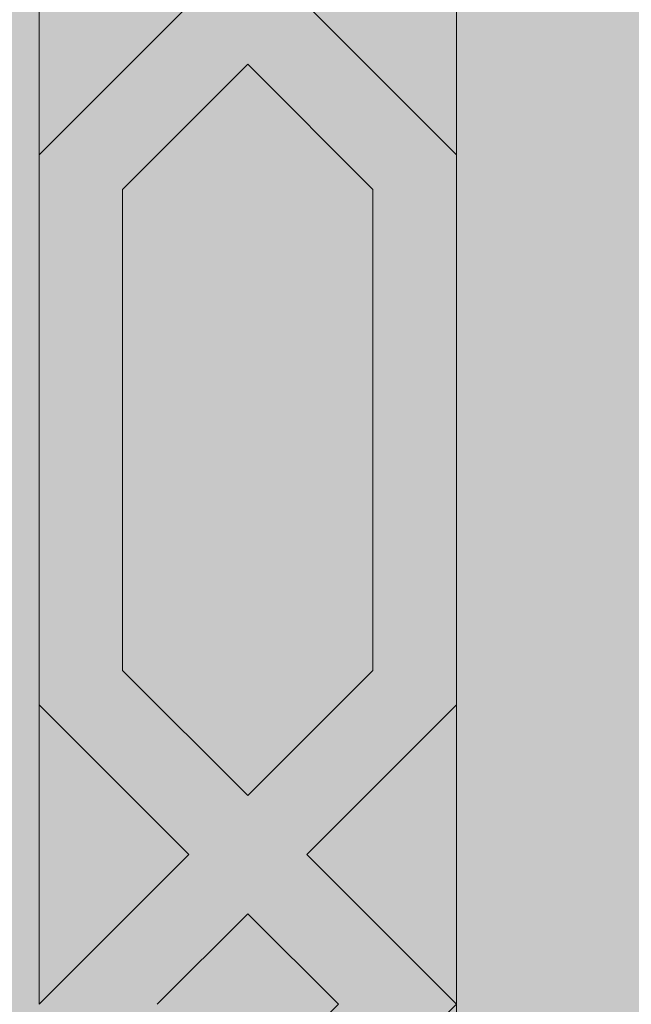
# Model space of a CAD drawing. Units: inches. Extents: x 844 to 2234, y 346 to 1084.
# Tile 14 of 93: x 1116.421 to 1118.29, y 696.22 to 699.229. Entities that reach past the tile are written whole.
import ezdxf

# ---------------------------------------------------------------- set-up
doc = ezdxf.new("R2010")
doc.units = ezdxf.units.IN
doc.header["$MEASUREMENT"] = 0
for name, color, linetype, lineweight in [('A-ANNO-DIMS', 2, 'Continuous', 18), ('furniture', 8, 'Continuous', 18), ('RA-AP-01$0$INT', 35, 'Continuous', 5)]:
    doc.layers.add(name, color=color, linetype=linetype, lineweight=lineweight)
doc.layers.add('RA-AP-01$0$FURN', color=3, linetype='Continuous')
doc.styles.get("Standard").update_dxf_attribs({"font": 'arial.ttf'})
doc.dimstyles.get("Standard").update_dxf_attribs({"dimtxt": 6, "dimasz": 3, "dimexe": 0.18, "dimexo": 0.0625, "dimgap": 0.09, "dimtad": 0, "dimtih": 1, "dimtoh": 1, "dimdec": 1, "dimzin": 0, "dimdsep": 46, "dimlunit": 3, "dimtxsty": 'Standard', "dimblk": 'ARCHTICK', "dimcen": 0.09, "dimadec": 0, "dimazin": 0, "dimtfac": 1, "dimtdec": 1, "dimtofl": 0, "dimtmove": 0, "dimatfit": 3, "dimfxl": 1, "dimtolj": 1, "dimtzin": 0, "dimarcsym": 0})

# ---------------------------------------------------------------- blocks, each defined once
blk = doc.blocks.new('A$C18D01794')
at = {"layer": 'RA-AP-01$0$INT'}
h = blk.add_hatch(color=256, dxfattribs=at)
h.paths.add_polyline_path([(4.35521, -6.15671), (4.35521, -8.05671), (5.45521, -8.05671), (5.45521, -6.15671)])
h.paths.add_polyline_path([(4.40521, -8.00671), (4.40521, -6.20671), (5.40521, -6.20671), (5.40521, -8.00671)], flags=16)
h = blk.add_hatch(color=256, dxfattribs=at)
h.paths.add_polyline_path([(4.46935, -7.07085), (4.50521, -7.035), (4.50521, -7.10671)])
h.paths.add_polyline_path([(4.45521, -7.085), (4.47692, -7.10671), (4.43349, -7.10671)])
h.paths.add_polyline_path([(4.40521, -7.035), (4.44106, -7.07085), (4.40521, -7.10671)])
h.paths.add_polyline_path([(4.42521, -6.91146), (4.45521, -6.88146), (4.48521, -6.91146), (4.48521, -7.02671), (4.45521, -7.05671), (4.42521, -7.02671)])
h.paths.add_polyline_path([(4.50521, -6.83146), (4.50521, -6.90318), (4.46935, -6.86732)])
h.paths.add_polyline_path([(4.42521, -6.70793), (4.45521, -6.67793), (4.48521, -6.70793), (4.48521, -6.82318), (4.45521, -6.85318), (4.42521, -6.82318)])
h.paths.add_polyline_path([(4.42521, -6.50439), (4.45521, -6.47439), (4.48521, -6.50439), (4.48521, -6.61964), (4.45521, -6.64964), (4.42521, -6.61964)])
h.paths.add_polyline_path([(4.46935, -6.66378), (4.50521, -6.62793), (4.50521, -6.69964)])
h.paths.add_polyline_path([(4.40521, -6.62793), (4.44106, -6.66378), (4.40521, -6.69964)])
h.paths.add_polyline_path([(4.40521, -6.42439), (4.44106, -6.46025), (4.40521, -6.49611)])
h.paths.add_polyline_path([(4.46935, -6.46025), (4.50521, -6.42439), (4.50521, -6.49611)])
h.paths.add_polyline_path([(4.42521, -6.30085), (4.45521, -6.27085), (4.48521, -6.30085), (4.48521, -6.41611), (4.45521, -6.44611), (4.42521, -6.41611)])
h.paths.add_polyline_path([(4.42521, -6.22671), (4.47106, -6.22671), (4.42521, -6.27257)])
h.paths.add_polyline_path([(4.49935, -6.22671), (4.63606, -6.22671), (4.66606, -6.25671), (4.63606, -6.28671), (4.49935, -6.28671), (4.46935, -6.25671)])
h.paths.add_polyline_path([(4.68021, -6.27085), (4.71606, -6.30671), (4.64435, -6.30671)])
h.paths.add_polyline_path([(4.64435, -6.20671), (4.71606, -6.20671), (4.68021, -6.24257)])
h.paths.add_polyline_path([(4.72435, -6.22671), (4.86106, -6.22671), (4.89106, -6.25671), (4.86106, -6.28671), (4.72435, -6.28671), (4.69435, -6.25671)])
h.paths.add_polyline_path([(4.90521, -6.27085), (4.94106, -6.30671), (4.86935, -6.30671)])
h.paths.add_polyline_path([(4.86935, -6.20671), (4.94106, -6.20671), (4.90521, -6.24257)])
h.paths.add_polyline_path([(4.94935, -6.22671), (5.08606, -6.22671), (5.11606, -6.25671), (5.08606, -6.28671), (4.94935, -6.28671), (4.91935, -6.25671)])
h.paths.add_polyline_path([(5.13021, -6.27085), (5.16606, -6.30671), (5.09435, -6.30671)])
h.paths.add_polyline_path([(5.09435, -6.20671), (5.16606, -6.20671), (5.13021, -6.24257)])
h.paths.add_polyline_path([(5.17435, -6.22671), (5.31106, -6.22671), (5.34106, -6.25671), (5.31106, -6.28671), (5.17435, -6.28671), (5.14435, -6.25671)])
h.paths.add_polyline_path([(5.32521, -6.30085), (5.35521, -6.27085), (5.38521, -6.30085), (5.38521, -6.41611), (5.35521, -6.44611), (5.32521, -6.41611)])
h.paths.add_polyline_path([(5.33935, -6.22671), (5.38521, -6.22671), (5.38521, -6.27257)])
h.paths.add_polyline_path([(5.32521, -6.50439), (5.35521, -6.47439), (5.38521, -6.50439), (5.38521, -6.61964), (5.35521, -6.64964), (5.32521, -6.61964)])
h.paths.add_polyline_path([(5.30521, -6.42439), (5.34106, -6.46025), (5.30521, -6.49611)])
h.paths.add_polyline_path([(5.36935, -6.46025), (5.40521, -6.42439), (5.40521, -6.49611)])
h.paths.add_polyline_path([(5.40521, -6.62793), (5.40521, -6.69964), (5.36935, -6.66378)])
h.paths.add_polyline_path([(5.30521, -6.62793), (5.34106, -6.66378), (5.30521, -6.69964)])
h.paths.add_polyline_path([(5.32521, -6.70793), (5.35521, -6.67793), (5.38521, -6.70793), (5.38521, -6.82318), (5.35521, -6.85318), (5.32521, -6.82318)])
h.paths.add_polyline_path([(5.30521, -6.83146), (5.34106, -6.86732), (5.30521, -6.90318)])
h.paths.add_polyline_path([(5.32521, -6.91146), (5.35521, -6.88146), (5.38521, -6.91146), (5.38521, -7.02671), (5.35521, -7.05671), (5.32521, -7.02671)])
h.paths.add_polyline_path([(5.40458, -6.83209, 0.001218), (5.40521, -6.83231), (5.40521, -6.90318), (5.36935, -6.86732)])
h.paths.add_polyline_path([(5.36935, -7.07085), (5.40521, -7.035), (5.40521, -7.10671)])
h.paths.add_polyline_path([(5.35521, -7.085), (5.37692, -7.10671), (5.33349, -7.10671)])
h.paths.add_polyline_path([(5.30521, -7.035), (5.34106, -7.07085), (5.30521, -7.10671)])
h = blk.add_hatch(color=256, dxfattribs=at)
h.paths.add_polyline_path([(4.50521, -6.62793), (4.46935, -6.66378), (4.50521, -6.69964), (4.50521, -6.83146), (4.46935, -6.86732), (4.50521, -6.90318), (4.50521, -7.035), (4.46935, -7.07085), (4.50521, -7.10671), (4.47692, -7.10671), (4.45521, -7.085), (4.43349, -7.10671), (4.40521, -7.10671), (4.44106, -7.07085), (4.40521, -7.035), (4.40521, -6.90318), (4.44106, -6.86732), (4.40521, -6.83146), (4.40521, -6.69964), (4.44106, -6.66378), (4.40521, -6.62793), (4.40521, -6.49611), (4.44106, -6.46025), (4.40521, -6.42439), (4.40521, -6.20671), (4.64435, -6.20671), (4.68021, -6.24257), (4.71606, -6.20671), (4.86935, -6.20671), (4.90521, -6.24257), (4.94106, -6.20671), (5.09435, -6.20671), (5.13021, -6.24257), (5.16606, -6.20671), (5.40521, -6.20671), (5.40521, -6.42439), (5.36935, -6.46025), (5.40521, -6.49611), (5.40521, -6.62793), (5.36935, -6.66378), (5.40521, -6.69964), (5.40521, -6.83146), (5.36935, -6.86732), (5.40521, -6.90318), (5.40521, -7.035), (5.36935, -7.07085), (5.40521, -7.10671), (5.37692, -7.10671), (5.35521, -7.085), (5.33349, -7.10671), (5.30521, -7.10671), (5.34106, -7.07085), (5.30521, -7.035), (5.30521, -6.90318), (5.34106, -6.86732), (5.30521, -6.83146), (5.30521, -6.69964), (5.34106, -6.66378), (5.30521, -6.62793), (5.30521, -6.49611), (5.34106, -6.46025), (5.30521, -6.42439), (5.30521, -6.30671), (5.16606, -6.30671), (5.13021, -6.27085), (5.09435, -6.30671), (4.94106, -6.30671), (4.90521, -6.27085), (4.86935, -6.30671), (4.71606, -6.30671), (4.68021, -6.27085), (4.64435, -6.30671), (4.50521, -6.30671), (4.50521, -6.42439), (4.46935, -6.46025), (4.50521, -6.49611)])
h.paths.add_polyline_path([(4.48521, -6.50439), (4.45521, -6.47439), (4.42521, -6.50439), (4.42521, -6.61964), (4.45521, -6.64964), (4.48521, -6.61964)], flags=16)
h.paths.add_polyline_path([(4.45521, -6.44611), (4.48521, -6.41611), (4.48521, -6.30085), (4.45521, -6.27085), (4.42521, -6.30085), (4.42521, -6.41611)], flags=16)
h.paths.add_polyline_path([(4.45521, -6.67793), (4.42521, -6.70793), (4.42521, -6.82318), (4.45521, -6.85318), (4.48521, -6.82318), (4.48521, -6.70793)], flags=16)
h.paths.add_polyline_path([(4.49935, -6.28671), (4.63606, -6.28671), (4.66606, -6.25671), (4.63606, -6.22671), (4.49935, -6.22671), (4.46935, -6.25671)], flags=16)
h.paths.add_polyline_path([(4.42521, -6.27257), (4.47106, -6.22671), (4.42521, -6.22671)], flags=16)
h.paths.add_polyline_path([(4.45521, -6.88146), (4.42521, -6.91146), (4.42521, -7.02671), (4.45521, -7.05671), (4.48521, -7.02671), (4.48521, -6.91146)], flags=16)
h.paths.add_polyline_path([(4.72435, -6.28671), (4.86106, -6.28671), (4.89106, -6.25671), (4.86106, -6.22671), (4.72435, -6.22671), (4.69435, -6.25671)], flags=16)
h.paths.add_polyline_path([(4.91935, -6.25671), (4.94935, -6.28671), (5.08606, -6.28671), (5.11606, -6.25671), (5.08606, -6.22671), (4.94935, -6.22671)], flags=16)
h.paths.add_polyline_path([(5.14435, -6.25671), (5.17435, -6.28671), (5.31106, -6.28671), (5.34106, -6.25671), (5.31106, -6.22671), (5.17435, -6.22671)], flags=16)
h.paths.add_polyline_path([(5.32521, -6.61964), (5.35521, -6.64964), (5.38521, -6.61964), (5.38521, -6.50439), (5.35521, -6.47439), (5.32521, -6.50439)], flags=16)
h.paths.add_polyline_path([(5.32521, -6.41611), (5.35521, -6.44611), (5.38521, -6.41611), (5.38521, -6.30085), (5.35521, -6.27085), (5.32521, -6.30085)], flags=16)
h.paths.add_polyline_path([(5.32521, -6.70793), (5.32521, -6.82318), (5.35521, -6.85318), (5.38521, -6.82318), (5.38521, -6.70793), (5.35521, -6.67793)], flags=16)
h.paths.add_polyline_path([(5.32521, -6.91146), (5.32521, -7.02671), (5.35521, -7.05671), (5.38521, -7.02671), (5.38521, -6.91146), (5.35521, -6.88146)], flags=16)
h.paths.add_polyline_path([(5.33935, -6.22671), (5.38521, -6.27257), (5.38521, -6.22671)], flags=16)
for points in [[(4.50521, -6.30671), (5.30521, -6.30671), (5.30521, -7.10671), (5.25521, -7.10671), (5.25521, -6.35671), (4.55521, -6.35671), (4.55521, -7.10671), (4.50521, -7.10671)], [(4.50521, -7.90671), (5.30521, -7.90671), (5.30521, -7.10671), (5.25521, -7.10671), (5.25521, -7.85671), (4.55521, -7.85671), (4.55521, -7.10671), (4.50521, -7.10671)], [(4.40521, -7.38196), (4.44106, -7.34611), (4.40521, -7.31025)]]:
    blk.add_hatch(color=256, dxfattribs=at).paths.add_polyline_path(points)
h = blk.add_hatch(color=256, dxfattribs=at)
h.paths.add_polyline_path([(4.50521, -7.5855), (4.46935, -7.54964), (4.50521, -7.51378), (4.50521, -7.38196), (4.46935, -7.34611), (4.50521, -7.31025), (4.50521, -7.17843), (4.46935, -7.14257), (4.50521, -7.10671), (4.47692, -7.10671), (4.45521, -7.12843), (4.43349, -7.10671), (4.40521, -7.10671), (4.44106, -7.14257), (4.40521, -7.17843), (4.40521, -7.31025), (4.44106, -7.34611), (4.40521, -7.38196), (4.40521, -7.51378), (4.44106, -7.54964), (4.40521, -7.5855), (4.40521, -7.71732), (4.44106, -7.75318), (4.40521, -7.78903), (4.40521, -8.00671), (4.64435, -8.00671), (4.68021, -7.97085), (4.71606, -8.00671), (4.86935, -8.00671), (4.90521, -7.97085), (4.94106, -8.00671), (5.09435, -8.00671), (5.13021, -7.97085), (5.16606, -8.00671), (5.40521, -8.00671), (5.40521, -7.78903), (5.36935, -7.75318), (5.40521, -7.71732), (5.40521, -7.5855), (5.36935, -7.54964), (5.40521, -7.51378), (5.40521, -7.38196), (5.36935, -7.34611), (5.40521, -7.31025), (5.40521, -7.17843), (5.36935, -7.14257), (5.40521, -7.10671), (5.37692, -7.10671), (5.35521, -7.12843), (5.33349, -7.10671), (5.30521, -7.10671), (5.34106, -7.14257), (5.30521, -7.17843), (5.30521, -7.31025), (5.34106, -7.34611), (5.30521, -7.38196), (5.30521, -7.51378), (5.34106, -7.54964), (5.30521, -7.5855), (5.30521, -7.71732), (5.34106, -7.75318), (5.30521, -7.78903), (5.30521, -7.90671), (5.16606, -7.90671), (5.13021, -7.94257), (5.09435, -7.90671), (4.94106, -7.90671), (4.90521, -7.94257), (4.86935, -7.90671), (4.71606, -7.90671), (4.68021, -7.94257), (4.64435, -7.90671), (4.50521, -7.90671), (4.50521, -7.78903), (4.46935, -7.75318), (4.50521, -7.71732)])
h.paths.add_polyline_path([(4.48521, -7.70903), (4.45521, -7.73903), (4.42521, -7.70903), (4.42521, -7.59378), (4.45521, -7.56378), (4.48521, -7.59378)], flags=16)
h.paths.add_polyline_path([(4.45521, -7.76732), (4.48521, -7.79732), (4.48521, -7.91257), (4.45521, -7.94257), (4.42521, -7.91257), (4.42521, -7.79732)], flags=16)
h.paths.add_polyline_path([(4.45521, -7.5355), (4.42521, -7.5055), (4.42521, -7.39025), (4.45521, -7.36025), (4.48521, -7.39025), (4.48521, -7.5055)], flags=16)
h.paths.add_polyline_path([(4.49935, -7.92671), (4.63606, -7.92671), (4.66606, -7.95671), (4.63606, -7.98671), (4.49935, -7.98671), (4.46935, -7.95671)], flags=16)
h.paths.add_polyline_path([(4.42521, -7.94085), (4.47106, -7.98671), (4.42521, -7.98671)], flags=16)
h.paths.add_polyline_path([(4.45521, -7.33196), (4.42521, -7.30196), (4.42521, -7.18671), (4.45521, -7.15671), (4.48521, -7.18671), (4.48521, -7.30196)], flags=16)
h.paths.add_polyline_path([(4.72435, -7.92671), (4.86106, -7.92671), (4.89106, -7.95671), (4.86106, -7.98671), (4.72435, -7.98671), (4.69435, -7.95671)], flags=16)
h.paths.add_polyline_path([(4.91935, -7.95671), (4.94935, -7.92671), (5.08606, -7.92671), (5.11606, -7.95671), (5.08606, -7.98671), (4.94935, -7.98671)], flags=16)
h.paths.add_polyline_path([(5.14435, -7.95671), (5.17435, -7.92671), (5.31106, -7.92671), (5.34106, -7.95671), (5.31106, -7.98671), (5.17435, -7.98671)], flags=16)
h.paths.add_polyline_path([(5.32521, -7.59378), (5.35521, -7.56378), (5.38521, -7.59378), (5.38521, -7.70903), (5.35521, -7.73903), (5.32521, -7.70903)], flags=16)
h.paths.add_polyline_path([(5.32521, -7.79732), (5.35521, -7.76732), (5.38521, -7.79732), (5.38521, -7.91257), (5.35521, -7.94257), (5.32521, -7.91257)], flags=16)
h.paths.add_polyline_path([(5.32521, -7.5055), (5.32521, -7.39025), (5.35521, -7.36025), (5.38521, -7.39025), (5.38521, -7.5055), (5.35521, -7.5355)], flags=16)
h.paths.add_polyline_path([(5.32521, -7.30196), (5.32521, -7.18671), (5.35521, -7.15671), (5.38521, -7.18671), (5.38521, -7.30196), (5.35521, -7.33196)], flags=16)
h.paths.add_polyline_path([(5.33935, -7.98671), (5.38521, -7.94085), (5.38521, -7.98671)], flags=16)
h = blk.add_hatch(color=256, dxfattribs=at)
h.paths.add_polyline_path([(4.46935, -7.14257), (4.50521, -7.17843), (4.50521, -7.10671)])
h.paths.add_polyline_path([(4.45521, -7.12843), (4.47692, -7.10671), (4.43349, -7.10671)])
h.paths.add_polyline_path([(4.40521, -7.17843), (4.44106, -7.14257), (4.40521, -7.10671)])
h.paths.add_polyline_path([(4.42521, -7.30196), (4.45521, -7.33196), (4.48521, -7.30196), (4.48521, -7.18671), (4.45521, -7.15671), (4.42521, -7.18671)])
h.paths.add_polyline_path([(4.50521, -7.38196), (4.50521, -7.31025), (4.46935, -7.34611)])
h.paths.add_polyline_path([(4.42521, -7.5055), (4.45521, -7.5355), (4.48521, -7.5055), (4.48521, -7.39025), (4.45521, -7.36025), (4.42521, -7.39025)])
h.paths.add_polyline_path([(4.42521, -7.70903), (4.45521, -7.73903), (4.48521, -7.70903), (4.48521, -7.59378), (4.45521, -7.56378), (4.42521, -7.59378)])
h.paths.add_polyline_path([(4.46935, -7.54964), (4.50521, -7.5855), (4.50521, -7.51378)])
h.paths.add_polyline_path([(4.40521, -7.5855), (4.44106, -7.54964), (4.40521, -7.51378)])
h.paths.add_polyline_path([(4.40521, -7.78903), (4.44106, -7.75318), (4.40521, -7.71732)])
h.paths.add_polyline_path([(4.46935, -7.75318), (4.50521, -7.78903), (4.50521, -7.71732)])
h.paths.add_polyline_path([(4.42521, -7.91257), (4.45521, -7.94257), (4.48521, -7.91257), (4.48521, -7.79732), (4.45521, -7.76732), (4.42521, -7.79732)])
h.paths.add_polyline_path([(4.42521, -7.98671), (4.47106, -7.98671), (4.42521, -7.94085)])
h.paths.add_polyline_path([(4.49935, -7.98671), (4.63606, -7.98671), (4.66606, -7.95671), (4.63606, -7.92671), (4.49935, -7.92671), (4.46935, -7.95671)])
h.paths.add_polyline_path([(4.68021, -7.94257), (4.71606, -7.90671), (4.64435, -7.90671)])
h.paths.add_polyline_path([(4.64435, -8.00671), (4.71606, -8.00671), (4.68021, -7.97085)])
h.paths.add_polyline_path([(4.72435, -7.98671), (4.86106, -7.98671), (4.89106, -7.95671), (4.86106, -7.92671), (4.72435, -7.92671), (4.69435, -7.95671)])
h.paths.add_polyline_path([(4.90521, -7.94257), (4.94106, -7.90671), (4.86935, -7.90671)])
h.paths.add_polyline_path([(4.86935, -8.00671), (4.94106, -8.00671), (4.90521, -7.97085)])
h.paths.add_polyline_path([(4.94935, -7.98671), (5.08606, -7.98671), (5.11606, -7.95671), (5.08606, -7.92671), (4.94935, -7.92671), (4.91935, -7.95671)])
h.paths.add_polyline_path([(5.13021, -7.94257), (5.16606, -7.90671), (5.09435, -7.90671)])
h.paths.add_polyline_path([(5.09435, -8.00671), (5.16606, -8.00671), (5.13021, -7.97085)])
h.paths.add_polyline_path([(5.17435, -7.98671), (5.31106, -7.98671), (5.34106, -7.95671), (5.31106, -7.92671), (5.17435, -7.92671), (5.14435, -7.95671)])
h.paths.add_polyline_path([(5.32521, -7.91257), (5.35521, -7.94257), (5.38521, -7.91257), (5.38521, -7.79732), (5.35521, -7.76732), (5.32521, -7.79732)])
h.paths.add_polyline_path([(5.33935, -7.98671), (5.38521, -7.98671), (5.38521, -7.94085)])
h.paths.add_polyline_path([(5.32521, -7.70903), (5.35521, -7.73903), (5.38521, -7.70903), (5.38521, -7.59378), (5.35521, -7.56378), (5.32521, -7.59378)])
h.paths.add_polyline_path([(5.30521, -7.78903), (5.34106, -7.75318), (5.30521, -7.71732)])
h.paths.add_polyline_path([(5.36935, -7.75318), (5.40521, -7.78903), (5.40521, -7.71732)])
h.paths.add_polyline_path([(5.40521, -7.5855), (5.40521, -7.51378), (5.36935, -7.54964)])
h.paths.add_polyline_path([(5.30521, -7.5855), (5.34106, -7.54964), (5.30521, -7.51378)])
h.paths.add_polyline_path([(5.32521, -7.5055), (5.35521, -7.5355), (5.38521, -7.5055), (5.38521, -7.39025), (5.35521, -7.36025), (5.32521, -7.39025)])
h.paths.add_polyline_path([(5.30521, -7.38196), (5.34106, -7.34611), (5.30521, -7.31025)])
h.paths.add_polyline_path([(5.32521, -7.30196), (5.35521, -7.33196), (5.38521, -7.30196), (5.38521, -7.18671), (5.35521, -7.15671), (5.32521, -7.18671)])
h.paths.add_polyline_path([(5.40458, -7.38134, -0.001218), (5.40521, -7.38111), (5.40521, -7.31025), (5.36935, -7.34611)])
h.paths.add_polyline_path([(5.36935, -7.14257), (5.40521, -7.17843), (5.40521, -7.10671)])
h.paths.add_polyline_path([(5.35521, -7.12843), (5.37692, -7.10671), (5.33349, -7.10671)])
h.paths.add_polyline_path([(5.30521, -7.17843), (5.34106, -7.14257), (5.30521, -7.10671)])
for p, q in [((4.46935, -7.07085), (4.50521, -7.10671)), ((4.45521, -7.085), (4.47692, -7.10671)), ((4.44106, -7.14257), (4.40521, -7.10671)), ((4.45521, -7.12843), (4.43349, -7.10671)), ((4.45521, -7.12843), (4.47692, -7.10671)), ((4.46935, -7.14257), (4.50521, -7.10671)), ((4.40521, -7.17843), (4.44106, -7.14257)), ((4.50521, -7.17843), (4.46935, -7.14257)), ((4.42521, -7.18671), (4.45521, -7.15671)), ((4.48521, -7.18671), (4.45521, -7.15671)), ((4.42521, -7.30196), (4.42521, -7.18671)), ((4.48521, -7.30196), (4.48521, -7.18671)), ((4.42521, -7.30196), (4.45521, -7.33196)), ((4.48521, -7.30196), (4.45521, -7.33196)), ((4.40521, -7.31025), (4.44106, -7.34611)), ((4.50521, -7.31025), (4.46935, -7.34611))]:
    blk.add_line(p, q, dxfattribs=at)
for points in [[(5.30521, -7.10671), (5.30521, -6.30671), (4.50521, -6.30671), (4.50521, -7.10671)], [(5.40521, -8.00671), (4.40521, -8.00671), (4.40521, -7.10671)], [(5.30521, -7.10671), (5.30521, -7.90671), (4.50521, -7.90671), (4.50521, -7.10671)]]:
    blk.add_lwpolyline(points, dxfattribs=at)
blk = doc.blocks.new('A$C5D2F253E')
at = {"layer": 'RA-AP-01$0$FURN', "xscale": -0.7999999999883585, "yscale": 0.7999999999883585, "zscale": 0.8, "rotation": 90}
blk.add_blockref('A$C18D01794', (-5.68776, 4.75792), dxfattribs=at)
blk = doc.blocks.new('_ArchTick')
at = {"color": 0, "linetype": 'ByBlock', "const_width": 0.15}
blk.add_lwpolyline([(-0.5, -0.5), (0.5, 0.5)], dxfattribs=at)
blk = doc.blocks.new('*D144')
at = {"layer": 'A-ANNO-DIMS', "color": 0, "lineweight": -2, "transparency": 16777216}
for p, q in [((1096.6159, 439.3733), (1096.6159, 1074.7433)), ((1143.1159, 492.3733), (1143.1159, 1074.7433)), ((1096.6159, 1074.5633), (1102.482, 1074.5633)), ((1143.1159, 1074.5633), (1137.2499, 1074.5633))]:
    blk.add_line(p, q, dxfattribs=at)
at = {"layer": 'Defpoints', "color": 0, "transparency": 16777216}
for p in [(1143.1159, 1074.5633), (1143.1159, 492.3108), (1096.6159, 439.3108)]:
    blk.add_point(p, dxfattribs=at)
at = {"layer": 'A-ANNO-DIMS', "color": 0, "lineweight": -2, "transparency": 16777216, "xscale": 3, "yscale": 3, "zscale": 3, "rotation": 180}
blk.add_blockref('_ArchTick', (1096.6159, 1074.5633), dxfattribs=at)
at = {"layer": 'A-ANNO-DIMS', "color": 0, "lineweight": -2, "transparency": 16777216, "xscale": 3, "yscale": 3, "zscale": 3}
blk.add_blockref('_ArchTick', (1143.1159, 1074.5633), dxfattribs=at)
at = {"layer": 'A-ANNO-DIMS', "color": 0, "transparency": 16777216, "insert": (1119.8659, 1074.5633), "char_height": 6, "attachment_point": 5}
blk.add_mtext('\\A1;3\'-10 1/2"', dxfattribs=at)

msp = doc.modelspace()

# ---------------------------------------------------------------- block references
at = {"layer": 'furniture', "xscale": 15.94108302203742, "yscale": 15.94108302203742, "zscale": 15.94108302203742, "rotation": 90}
msp.add_blockref('A$C5D2F253E', (1136.1478, 696.2585), dxfattribs=at)

# ---------------------------------------------------------------- dimensions: what is measured, and where the dimension line sits
at = {"layer": 'A-ANNO-DIMS'}
dim = msp.add_linear_dim(base=(1143.1159, 1074.5633), p1=(1096.6159, 439.3108), p2=(1143.1159, 492.3108), dimstyle='Standard', override={"dimdec": 1, "dimlfac": 1, "dimrnd": 0, "dimzin": 1, "dimdsep": 46, "dimlunit": 4, "dimfrac": 2}, dxfattribs=at)
dim.commit()
dim.dimension.update_dxf_attribs({"geometry": '*D144', "text_midpoint": (1119.8659, 1074.5633)})

doc.saveas('drawing.dxf')
